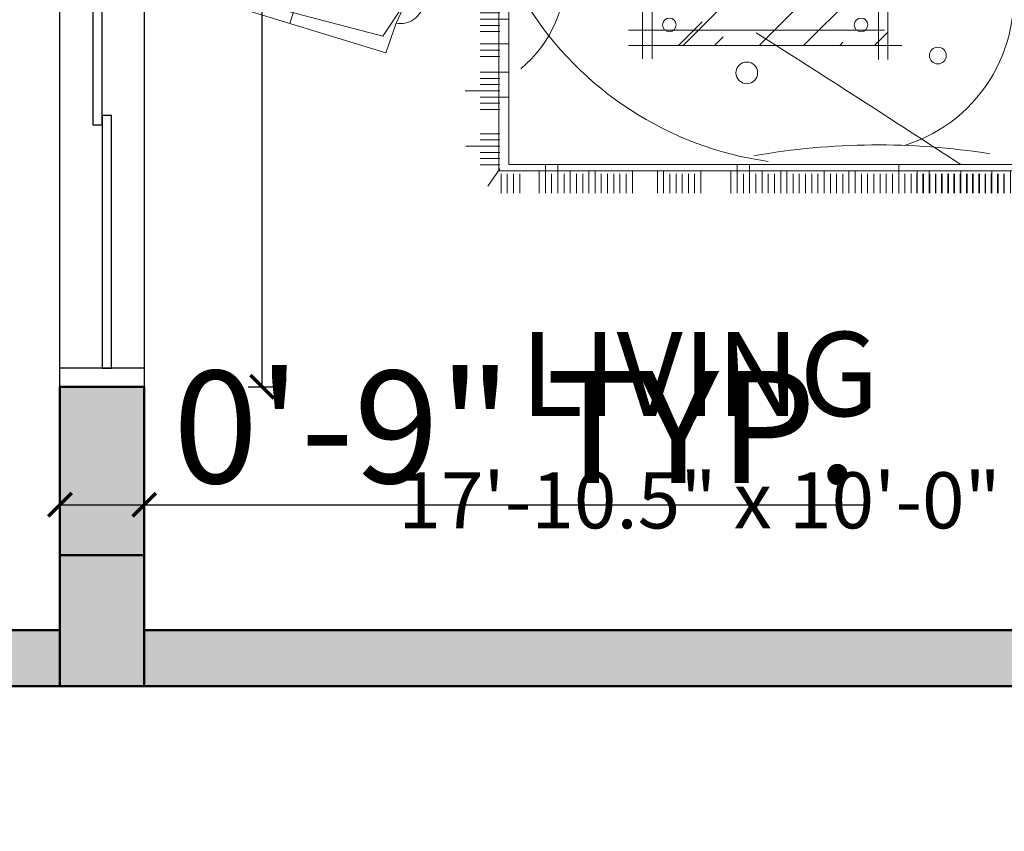
# Model space of a CAD drawing. Units: inches. Extents: x 375 to 1122, y 27 to 1069.
# Tile 4 of 155: x 494 to 599, y 313 to 400. Entities that reach past the tile are written whole.
import ezdxf

# ---------------------------------------------------------------- set-up
doc = ezdxf.new("R2010")
doc.units = ezdxf.units.IN
for name, color, linetype, lineweight in [('A-ANNO-DIMS', 2, 'Continuous', 18), ('A-AREA-IDEN', 7, 'Continuous', 18), ('A-COLS-PATT', 10, 'Continuous', 13), ('A-WALL-PATT', 252, 'Continuous', 13), ('Columns', 10, 'Continuous', 50), ('Doors', 150, 'Continuous', 25), ('Furniture', 30, 'Continuous', 18), ('Walls', 250, 'Continuous', 50)]:
    doc.layers.add(name, color=color, linetype=linetype, lineweight=lineweight)
doc.styles.get("Standard").update_dxf_attribs({"font": 'arial.ttf'})
doc.dimstyles.new('ISO-25', dxfattribs={"dimtxt": 12, "dimasz": 2.5, "dimexe": 1.5, "dimexo": 1.5, "dimtad": 1, "dimdec": 1, "dimlunit": 3, "dimtxsty": 'Standard', "dimblk": 'ARCHTICK', "dimcen": 2.5, "dimadec": 0, "dimazin": 0, "dimtfac": 1, "dimtdec": 1, "dimtmove": 0, "dimatfit": 3, "dimfxl": 1.5, "dimfxlon": 1, "dimarcsym": 0})

# ---------------------------------------------------------------- blocks, each defined once
blk = doc.blocks.new('A$C4DC51D13')
for p, q in [((3265.3, 2996.2), (1188.4, 2996.2)), ((1895.2, 2134), (1895.2, 2996.2)), ((2559.6, 2996.2), (2559.6, 2617.8)), ((1188.4, 2962.7), (1862.1, 2962.7)), ((1862.1, 2134), (1862.1, 2962.7)), ((1928.3, 2961.6), (2524.2, 2961.6)), ((1928.3, 2134), (1928.3, 2961.6)), ((2524.2, 2961.6), (2524.2, 2658.6)), ((2590.4, 2962.7), (2590.4, 2654.5)), ((3265.3, 2962.7), (2590.4, 2962.7)), ((277.4, 2939.6), (277.4, 2141.8)), ((943, 2103.5), (943, 2936.7)), ((1018.2, 2892.3), (232.2, 2892.3)), ((304, 2865.7), (304, 2253.3)), ((916.4, 2865.7), (304, 2865.7)), ((916.4, 2253.3), (916.4, 2865.7)), ((1290.4, 2664.8), (1028, 2870.9)), ((3163.3, 2664.8), (3425.7, 2870.9)), ((3778.5, 2897), (3631.2, 2747.3)), ((4008.9, 2375.5), (3778.5, 2897)), ((4156.2, 2525.2), (3778.5, 2897)), ((1022.9, 2163.8), (1022.9, 2830.3)), ((1056, 2830.3), (1081, 2194.8)), ((3397.7, 2830.3), (3364.5, 2194.8)), ((3430.8, 2163.8), (3430.8, 2830.3)), ((423.7, 2370.8), (776.6, 2723.7)), ((427.4, 2727.4), (772.8, 2367.1)), ((531.8, 2670.2), (531.8, 2717)), ((536, 2672.5), (536, 2718.7)), ((540.2, 2674.6), (540.2, 2720.2)), ((544.4, 2676.5), (544.4, 2721.6)), ((548.7, 2678.2), (548.7, 2722.9)), ((650.1, 2678.8), (650.1, 2723.3)), ((654.3, 2677.1), (654.3, 2722)), ((658.6, 2675.2), (658.6, 2720.7)), ((662.8, 2673.2), (662.8, 2719.2)), ((667, 2671), (667, 2717.6)), ((668.5, 2670.2), (668.5, 2717)), ((4008.9, 2375.5), (3631.2, 2747.3)), ((476.8, 2615), (476.8, 2682.5)), ((481, 2622.2), (481, 2686.2)), ((485.3, 2628.5), (485.3, 2689.7)), ((489.5, 2634.2), (489.5, 2693)), ((493.7, 2639.3), (493.7, 2696.1)), ((497.9, 2644), (497.9, 2699.1)), ((502.2, 2648.3), (502.2, 2701.8)), ((506.4, 2652.2), (506.4, 2704.4)), ((510.6, 2655.8), (510.6, 2706.9)), ((514.9, 2659.2), (514.9, 2709.2)), ((519.1, 2662.3), (519.1, 2711.3)), ((523.3, 2665.1), (523.3, 2713.4)), ((527.5, 2667.8), (527.5, 2715.2)), ((671.2, 2668.6), (671.2, 2715.9)), ((672.7, 2667.8), (672.7, 2715.2)), ((675.5, 2666.1), (675.5, 2714)), ((676.9, 2665.1), (676.9, 2713.4)), ((679.7, 2663.3), (679.7, 2712)), ((681.1, 2662.3), (681.1, 2711.3)), ((683.9, 2660.3), (683.9, 2709.9)), ((685.4, 2659.2), (685.4, 2709.2)), ((688.1, 2657), (688.1, 2707.7)), ((689.6, 2655.8), (689.6, 2706.9)), ((692.4, 2653.5), (692.4, 2705.3)), ((693.8, 2652.2), (693.8, 2704.4)), ((696.6, 2649.6), (696.6, 2702.7)), ((698, 2648.3), (698, 2701.8)), ((700.8, 2645.5), (700.8, 2700)), ((702.3, 2644), (702.3, 2699.1)), ((705, 2641), (705, 2697.2)), ((706.5, 2639.3), (706.5, 2696.1)), ((709.3, 2636), (709.3, 2694.1)), ((710.7, 2634.2), (710.7, 2693)), ((713.5, 2630.5), (713.5, 2690.9)), ((714.9, 2628.5), (714.9, 2689.7)), ((717.7, 2624.4), (717.7, 2687.4)), ((719.2, 2622.2), (719.2, 2686.2)), ((722, 2617.6), (722, 2683.8)), ((723.4, 2615), (723.4, 2682.5)), ((726.2, 2609.7), (726.2, 2679.9)), ((446.1, 2646.1), (500, 2646.1)), ((447.2, 2446.7), (447.2, 2647.8)), ((448.9, 2650.4), (504.4, 2650.4)), ((451.5, 2440.6), (451.5, 2654)), ((451.9, 2654.6), (509.2, 2654.6)), ((455.1, 2658.8), (514.4, 2658.8)), ((455.7, 2434.9), (455.7, 2659.6)), ((458.4, 2663.1), (520.2, 2663.1)), ((459.9, 2558.8), (459.9, 2664.9)), ((462, 2667.3), (526.7, 2667.3)), ((464.1, 2583.3), (464.1, 2669.7)), ((465.8, 2671.5), (534.1, 2671.5)), ((468.4, 2596.6), (468.4, 2674.3)), ((469.8, 2675.7), (542.8, 2675.7)), ((472.6, 2606.7), (472.6, 2678.5)), ((489.5, 2667.3), (489.5, 2633.5)), ((657.4, 2675.7), (730.4, 2675.7)), ((734.5, 2671.5), (666.1, 2671.5)), ((666.1, 2671.5), (734.5, 2671.5)), ((738.2, 2667.3), (673.5, 2667.3)), ((673.5, 2667.3), (738.2, 2667.3)), ((741.8, 2663.1), (680, 2663.1)), ((680, 2663.1), (741.8, 2663.1)), ((745.2, 2658.8), (685.8, 2658.8)), ((685.8, 2658.8), (745.2, 2658.8)), ((748.3, 2654.6), (691, 2654.6)), ((691, 2654.6), (748.3, 2654.6)), ((751.3, 2650.4), (695.8, 2650.4)), ((695.8, 2650.4), (751.3, 2650.4)), ((754.1, 2646.1), (700.2, 2646.1)), ((700.2, 2646.1), (754.1, 2646.1)), ((727.6, 2606.7), (727.6, 2678.5)), ((730.4, 2600.3), (730.4, 2675.7)), ((731.9, 2596.6), (731.9, 2674.3)), ((734.6, 2588.4), (734.6, 2671.3)), ((736.1, 2583.3), (736.1, 2669.7)), ((738.9, 2570.4), (738.9, 2666.6)), ((740.3, 2558.8), (740.3, 2664.9)), ((743.1, 2433.1), (743.1, 2661.5)), ((744.5, 2434.9), (744.5, 2659.6)), ((747.3, 2438.6), (747.3, 2656)), ((748.8, 2440.6), (748.8, 2654)), ((751.5, 2444.5), (751.5, 2650)), ((753, 2446.7), (753, 2647.8)), ((755.8, 2451.1), (755.8, 2643.5)), ((1283.3, 2574.2), (1290.4, 2664.8)), ((1290.4, 2664.8), (1894.7, 2664.8)), ((1895.2, 2663.7), (2557.3, 2663.7)), ((2603.6, 2664.8), (2559, 2664.8)), ((3163.3, 2664.8), (2764.7, 2664.8)), ((3170.4, 2574.2), (3163.3, 2664.8)), ((3631.7, 2676.6), (3938.2, 2375)), ((427.5, 2608.1), (473.3, 2608.1)), ((429.1, 2612.3), (475.4, 2612.3)), ((430.3, 2479), (430.3, 2615.5)), ((430.7, 2616.6), (477.7, 2616.6)), ((432.5, 2620.8), (480.2, 2620.8)), ((434.5, 2469.3), (434.5, 2625.2)), ((434.5, 2625), (482.9, 2625)), ((436.5, 2629.2), (485.8, 2629.2)), ((438.7, 2633.5), (488.9, 2633.5)), ((438.8, 2460.9), (438.8, 2633.6)), ((441, 2637.7), (492.3, 2637.7)), ((443, 2453.4), (443, 2641.1)), ((443.5, 2641.9), (496, 2641.9)), ((756.7, 2641.9), (704.2, 2641.9)), ((704.2, 2641.9), (756.7, 2641.9)), ((759.2, 2637.7), (707.9, 2637.7)), ((707.9, 2637.7), (759.2, 2637.7)), ((761.5, 2633.5), (711.3, 2633.5)), ((711.3, 2633.5), (761.5, 2633.5)), ((763.7, 2629.2), (714.4, 2629.2)), ((714.4, 2629.2), (763.7, 2629.2)), ((765.8, 2625), (717.3, 2625)), ((767.7, 2620.8), (720, 2620.8)), ((769.5, 2616.6), (722.5, 2616.6)), ((771.1, 2612.3), (724.8, 2612.3)), ((772.7, 2608.1), (726.9, 2608.1)), ((757.2, 2453.4), (757.2, 2641.1)), ((760, 2458.3), (760, 2636.3)), ((761.4, 2460.9), (761.4, 2633.6)), ((764.2, 2466.3), (764.2, 2628.2)), ((765.7, 2469.3), (765.7, 2625.2)), ((1798, 2530.2), (1812.1, 2637.9)), ((418.5, 2570.1), (461.3, 2570.1)), ((419.1, 2574.3), (462.1, 2574.3)), ((419.8, 2578.5), (462.9, 2578.5)), ((420.6, 2582.7), (464, 2582.7)), ((421.5, 2587), (465.2, 2587)), ((422.5, 2591.2), (466.5, 2591.2)), ((423.6, 2595.4), (467.9, 2595.4)), ((424.8, 2599.7), (469.6, 2599.7)), ((426.1, 2603.9), (471.3, 2603.9)), ((426.1, 2490.7), (426.1, 2603.9)), ((774.1, 2603.9), (728.9, 2603.9)), ((775.4, 2599.7), (730.7, 2599.7)), ((776.6, 2595.4), (732.3, 2595.4)), ((777.7, 2591.2), (733.7, 2591.2)), ((778.7, 2587), (735.1, 2587)), ((779.6, 2582.7), (736.2, 2582.7)), ((780.4, 2578.5), (737.3, 2578.5)), ((781.1, 2574.3), (738.2, 2574.3)), ((781.7, 2570.1), (738.9, 2570.1)), ((1895.5, 2582.2), (1932.3, 2494.6)), ((417.1, 2548.9), (459.4, 2548.9)), ((417.1, 2544.7), (459.5, 2544.7)), ((417.2, 2553.2), (459.6, 2553.2)), ((417.2, 2540.5), (459.6, 2540.5)), ((417.4, 2557.4), (459.8, 2557.4)), ((417.5, 2536.3), (459.9, 2536.3)), ((417.7, 2561.6), (460.2, 2561.6)), ((417.8, 2532), (460.3, 2532)), ((418.1, 2565.8), (460.7, 2565.8)), ((459.9, 2429.7), (459.9, 2535.7)), ((782.2, 2565.8), (739.6, 2565.8)), ((782.5, 2532), (740, 2532)), ((782.5, 2561.6), (740.1, 2561.6)), ((740.3, 2429.7), (740.3, 2535.7)), ((782.8, 2557.4), (740.4, 2557.4)), ((782.8, 2536.3), (740.4, 2536.3)), ((783, 2540.5), (740.6, 2540.5)), ((783, 2553.2), (740.7, 2553.2)), ((783.1, 2548.9), (740.8, 2548.9)), ((783.1, 2544.7), (740.8, 2544.7)), ((1022.9, 2554.4), (1249.6, 2554.4)), ((2559, 2535.8), (2557.3, 2535.8)), ((3430.8, 2554.4), (3204.1, 2554.4)), ((418.2, 2527.8), (460.8, 2527.8)), ((418.7, 2523.6), (461.4, 2523.6)), ((419.3, 2519.4), (462.2, 2519.4)), ((781, 2519.4), (738, 2519.4)), ((781.6, 2523.6), (738.8, 2523.6)), ((782.1, 2527.8), (739.4, 2527.8)), ((1200, 2520.5), (1251.9, 2440.8)), ((3253.7, 2520.5), (3201.8, 2440.8)), ((4008.9, 2375.5), (4156.2, 2525.2)), ((1243.2, 2146.7), (1272.2, 2431.8)), ((3210.5, 2146.7), (3181.5, 2431.8)), ((304, 2253.3), (916.4, 2253.3)), ((242.9, 2226.7), (1018.2, 2226.7)), ((1145.1, 2159.3), (1022.9, 2163.8)), ((1081, 2194.8), (1243.2, 2146.7)), ((1145.1, 2159.3), (1243.2, 2146.7)), ((2590.4, 2164.3), (2590.4, 2134)), ((3364.5, 2194.8), (3210.5, 2146.7)), ((3308.6, 2159.3), (3210.5, 2146.7)), ((3308.6, 2159.3), (3430.8, 2163.8)), ((498.8, 1837.1), (382.1, 2139.5)), ((1040.3, 1942.9), (421.2, 2132.6)), ((1244.8, 2113), (1243.2, 2146.7)), ((3208.9, 2113), (3210.5, 2146.7)), ((411.8, 2101.9), (992.6, 1890.2)), ((1839.5, 2113), (1244.8, 2113)), ((2308.5, 2111.9), (1950.4, 2111.9)), ((2614.2, 2113), (3208.9, 2113)), ((677.4, 2054.1), (612.9, 1843.6)), ((1839.5, 2079.9), (1244.8, 2079.9)), ((2322.1, 2078.8), (1950.4, 2078.8)), ((2614.2, 2079.9), (3208.9, 2079.9)), ((220.3, 2026), (19.3, 1370.1)), ((251.1, 2016.6), (37.1, 1314.7)), ((1009.7, 1828.1), (1040.3, 1942.9)), ((658.5, 1880), (717.8, 1809.1)), ((992.6, 1890.2), (993.4, 1733.4)), ((498.8, 1837.1), (341.4, 1323.6)), ((584.9, 1817.9), (498.8, 1837.1)), ((1009.7, 1828.1), (993.4, 1733.4)), ((1158.3, 1784.3), (1158.3, 1858.2)), ((1181.8, 1784.3), (1181.8, 1858.2)), ((1205.3, 1784.3), (1205.3, 1858.2)), ((1228.8, 1784.3), (1228.8, 1858.2)), ((1252.2, 1784.3), (1252.2, 1858.2)), ((1319.4, 1784.3), (1319.4, 1858.2)), ((1342.9, 1784.3), (1342.9, 1858.2)), ((1366.3, 1784.3), (1366.3, 1858.2)), ((1389.8, 1784.3), (1389.8, 1858.2)), ((1413.3, 1784.3), (1413.3, 1858.2)), ((1436.8, 1784.3), (1436.8, 1858.2)), ((1460.2, 1784.3), (1460.2, 1858.2)), ((1483.7, 1784.3), (1483.7, 1858.2)), ((1507.2, 1784.3), (1507.2, 1858.2)), ((1530.7, 1784.3), (1530.7, 1858.2)), ((1554.1, 1784.3), (1554.1, 1858.2)), ((1577.6, 1784.3), (1577.6, 1858.2)), ((1714.2, 1784.3), (1714.2, 1858.2)), ((1737.6, 1784.3), (1737.6, 1858.2)), ((1761.1, 1784.3), (1761.1, 1858.2)), ((1784.6, 1784.3), (1784.6, 1858.2)), ((1808.1, 1784.3), (1808.1, 1858.2)), ((1831.5, 1784.3), (1831.5, 1858.2)), ((1855, 1784.3), (1855, 1858.2)), ((1878.5, 1784.3), (1878.5, 1858.2)), ((1902, 1784.3), (1902, 1858.2)), ((2050.7, 1784.3), (2050.7, 1858.2)), ((2074.2, 1784.3), (2074.2, 1858.2)), ((2097.7, 1784.3), (2097.7, 1858.2)), ((2121.1, 1784.3), (2121.1, 1858.2)), ((2144.6, 1784.3), (2144.6, 1858.2)), ((2168.1, 1784.3), (2168.1, 1858.2)), ((2191.6, 1782.4), (2191.6, 1856.3)), ((2215, 1785.7), (2215, 1832.3)), ((2238.5, 1785.1), (2238.5, 1859)), ((2262, 1784.3), (2262, 1858.2)), ((2285.4, 1784.3), (2285.4, 1858.2)), ((2543.7, 1784.3), (2543.7, 1858.2)), ((2567.1, 1784.3), (2567.1, 1858.2)), ((2590.6, 1784.3), (2590.6, 1858.2)), ((2614.1, 1784.3), (2614.1, 1858.2)), ((2661, 1784.3), (2661, 1858.2)), ((2684.5, 1784.3), (2684.5, 1858.2)), ((2708, 1772.3), (2708, 1858.2)), ((2731.5, 1784.3), (2731.5, 1858.2)), ((2754.9, 1784.3), (2754.9, 1858.2)), ((2778.4, 1784.3), (2778.4, 1858.2)), ((2801.9, 1784.3), (2801.9, 1858.2)), ((2825.4, 1784.3), (2825.4, 1858.2)), ((2848.8, 1784.3), (2848.8, 1858.2)), ((2872.3, 1784.3), (2872.3, 1858.2)), ((2895.8, 1784.3), (2895.8, 1858.2)), ((2919.3, 1784.3), (2919.3, 1858.2)), ((2942.7, 1784.3), (2942.7, 1858.2)), ((2966.2, 1744.8), (2966.2, 1858.2)), ((2989.7, 1784.3), (2989.7, 1858.2)), ((3013.2, 1772.3), (3013.2, 1858.2)), ((3036.6, 1784.3), (3036.6, 1858.2)), ((3060.1, 1784.3), (3060.1, 1858.2)), ((3083.6, 1784.3), (3083.6, 1858.2)), ((993.4, 1733.4), (720.4, 1787.6)), ((1166.1, 1769.7), (1091.8, 1794.5)), ((1158.3, 1821.3), (1158.5, 487.7)), ((1162.1, 1754.9), (1088.2, 1754.9)), ((3248.4, 1772.3), (1158.5, 1772.3)), ((3248.4, 487.7), (3248.4, 1772.3)), ((3248.8, 1760.8), (3322.7, 1760.8)), ((1024.2, 1722.3), (842.3, 1125.2)), ((873.1, 1115.8), (1055, 1712.9)), ((1024.2, 1722.3), (993.4, 1733.4)), ((1162.1, 1741.1), (1088.2, 1741.1)), ((1162.1, 1717.6), (1088.2, 1717.6)), ((1196, 511), (1196, 1744.8)), ((1196, 1744.8), (3215.6, 1744.8)), ((3215.6, 511), (3215.6, 1744.8)), ((3248.8, 1737.3), (3322.7, 1737.3)), ((3248.8, 1713.8), (3322.7, 1713.8)), ((3600.6, 1621.7), (3605.1, 1743.8)), ((3605.1, 1743.8), (4271.6, 1743.8)), ((3995.7, 1743.8), (3995.7, 1517.1)), ((4106.1, 1476.4), (4312.2, 1738.8)), ((1162.1, 1708), (1088.2, 1708)), ((1162.1, 1684.5), (1088.2, 1684.5)), ((3248.8, 1690.4), (3322.7, 1690.4)), ((3636.1, 1685.8), (3588, 1523.6)), ((4271.6, 1710.7), (3636.1, 1685.8)), ((3248.8, 1666.9), (3322.7, 1666.9)), ((3248.8, 1643.4), (3322.7, 1643.4)), ((3248.8, 1619.9), (3322.7, 1619.9)), ((3600.6, 1621.7), (3588, 1523.6)), ((4404, 1578.3), (4404, 904.6)), ((4437.5, 165.9), (4437.5, 1578.3)), ((1701.7, 1530), (1701.7, 911.2)), ((1162.1, 1492.9), (1088.2, 1492.9)), ((2593.1, 907.9), (2593.1, 1490.3)), ((2629.1, 907.9), (2629.1, 1503.1)), ((3248.8, 1513.8), (3322.7, 1513.8)), ((3248.8, 1513.3), (3322.7, 1513.3)), ((3248.8, 1490.4), (3322.7, 1490.4)), ((3248.8, 1489.9), (3322.7, 1489.9)), ((3521.2, 1130.7), (3521.2, 1521.9)), ((3554.3, 1131.4), (3554.3, 1521.9)), ((3588, 1523.6), (3873.1, 1494.5)), ((1162.1, 1483.3), (1088.2, 1483.3)), ((1162.1, 1459.8), (1088.2, 1459.8)), ((1737.7, 1483.1), (1737.7, 911.2)), ((3248.8, 1466.9), (3322.7, 1466.9)), ((4015.5, 1483.4), (4106.1, 1476.4)), ((4106.1, 1476.4), (4106.1, 872.1)), ((1162.1, 1446), (1088.2, 1446)), ((2674.6, 1449.9), (1641, 1449.9)), ((1888.1, 1449.9), (1701.7, 1263.5)), ((1856.2, 1449.9), (1701.7, 1295.4)), ((1715.1, 1449.9), (1701.7, 1436.5)), ((2343.3, 1449.9), (1855.3, 961.9)), ((2629.1, 1449), (2142, 961.9)), ((2325.1, 1449.9), (2154.2, 1279.1)), ((2461.6, 1449.9), (2177, 1165.3)), ((3248.8, 1443.4), (3322.7, 1443.4)), ((3248.8, 1419.9), (3322.7, 1419.9)), ((1162.1, 1412.8), (1088.2, 1412.8)), ((1162.1, 1399), (1088.2, 1399)), ((2674.6, 1413.9), (1641, 1413.9)), ((3250, 1407.8), (3519, 1407.8)), ((6.3, 1324.2), (19.3, 1370.2)), ((479.3, 1327.3), (375.2, 1344.9)), ((1162.1, 1375.5), (1088.2, 1375.5)), ((1162.1, 1352.1), (1088.2, 1352.1)), ((1162.1, 1342.9), (1088.2, 1342.9)), ((1162.1, 1342.4), (1088.2, 1342.4)), ((3248.8, 1359), (3322.7, 1359)), ((342.8, 1324.6), (76.7, 1139.6)), ((843, 1127.6), (342.8, 1324.6)), ((1162.1, 1319.4), (1088.2, 1319.4)), ((1162.1, 1318.9), (1088.2, 1318.9)), ((3248.8, 990.8), (3248.4, 1328.4)), ((3248.8, 1312.1), (3322.7, 1312.1)), ((3250, 1317.8), (3519, 1317.8)), ((369.2, 1044.8), (442.9, 1285.2)), ((1162.1, 1296), (1088.2, 1296)), ((1162.1, 1295.5), (1088.2, 1295.5)), ((1196, 1272.5), (1088.2, 1272.5)), ((1162.1, 1272), (1088.2, 1272)), ((2629.1, 1280.5), (2310.5, 961.9)), ((3248.8, 1302.3), (3322.7, 1302.3)), ((1162.1, 1249), (1088.2, 1249)), ((1162.1, 1248.5), (1088.2, 1248.5)), ((3248.8, 1249), (3322.7, 1249)), ((3248.8, 1248.5), (3322.7, 1248.5)), ((3248.8, 1239.3), (3322.7, 1239.3)), ((3248.8, 1238.8), (3322.7, 1238.8)), ((1162.1, 1225.5), (1088.2, 1225.5)), ((1162.1, 1202.1), (1088.2, 1202.1)), ((3248.8, 1225.5), (3322.7, 1225.5)), ((3248.8, 1202.1), (3322.7, 1202.1)), ((122.4, 1154.1), (719.7, 996.3)), ((1196, 1178.6), (1088.2, 1178.6)), ((1162.1, 1155.1), (1088.2, 1155.1)), ((1728.6, 1158.4), (1701.7, 1131.5)), ((3248.8, 1178.6), (3322.7, 1178.6)), ((3248.8, 1155.1), (3322.7, 1155.1)), ((732, 933.5), (112.9, 1123.3)), ((719.7, 996.3), (810.6, 1133.2)), ((771, 1045.7), (810.6, 1133.2)), ((842.3, 1125.2), (810.6, 1133.2)), ((1162.1, 1131.6), (1088.2, 1131.6)), ((3248.8, 1131.6), (3322.7, 1131.6)), ((1162.1, 1108.2), (1088.2, 1108.2)), ((1162.1, 1084.7), (1088.2, 1084.7)), ((3248.8, 1108.2), (3322.7, 1108.2)), ((771, 1045.7), (732, 933.5)), ((1196, 1061.2), (1088.2, 1061.2)), ((1926.6, 1051.5), (1837.1, 961.9)), ((1162.1, 1037.7), (1088.2, 1037.7)), ((1162.1, 1014.3), (1088.2, 1014.3)), ((1648.3, 1019.6), (2616.7, 1019.6)), ((2629.1, 1012), (2579, 961.9)), ((3248.8, 1014.3), (3322.7, 1014.3)), ((2006.3, 994.6), (1973.6, 961.9)), ((2459.2, 974.1), (2447, 961.9)), ((3248.8, 990.8), (3322.7, 990.8)), ((1196, 967.3), (1088.2, 967.3)), ((1162.1, 943.8), (1088.2, 943.8)), ((1648.3, 961.9), (2681.9, 961.9)), ((3248.8, 967.3), (3322.7, 967.3)), ((3248.8, 943.8), (3322.7, 943.8)), ((1162.1, 920.4), (1088.2, 920.4)), ((3248.8, 920.4), (3322.7, 920.4)), ((4097.4, 904.6), (4404, 904.6)), ((1196, 860.5), (1088.2, 860.5)), ((4106.1, 871.5), (4437.5, 871.5)), ((1162.1, 837), (1088.2, 837)), ((4404, 840.7), (4110.5, 840.7)), ((4404, 165.9), (4404, 840.7)), ((1162.1, 790), (1031.8, 790)), ((1162.1, 813.5), (1088.2, 813.5)), ((3521.2, 816.9), (3521.2, 222.3)), ((3554.3, 816.9), (3554.3, 222.3)), ((1196, 766.6), (1088.2, 766.6)), ((1162.1, 743.1), (1088.2, 743.1)), ((1162.1, 719.6), (1088.2, 719.6)), ((4106.1, 267.8), (4106.1, 666.5)), ((1162.1, 627.8), (1088.2, 627.8)), ((1162.1, 604.4), (1088.2, 604.4)), ((3248.8, 627.8), (3322.7, 627.8)), ((3248.8, 604.4), (3322.7, 604.4)), ((1162.1, 580.9), (1034.2, 580.9)), ((3248.8, 580.9), (3322.7, 580.9)), ((1162.1, 557.4), (1088.2, 557.4)), ((1162.1, 533.9), (1088.2, 533.9)), ((3248.8, 557.4), (3322.7, 557.4)), ((3248.8, 533.9), (3322.7, 533.9)), ((1162.1, 510.5), (1088.2, 510.5)), ((1162, 495.1), (1116.6, 429)), ((1158.5, 487.7), (3248.4, 487.7)), ((3215.6, 511), (1196, 511)), ((1311.1, 487.7), (1311.1, 402.4)), ((1334.6, 511), (1334.6, 402.4)), ((1381.6, 511), (1381.6, 402.4)), ((1428.5, 487.7), (1428.5, 402.4)), ((1498.9, 487.7), (1498.9, 402.4)), ((1522.4, 487.7), (1522.4, 402.4)), ((1663.3, 487.7), (1663.3, 402.4)), ((1757.8, 487.7), (1757.8, 402.4)), ((1781.3, 487.7), (1781.3, 402.4)), ((1922.1, 487.7), (1922.1, 402.4)), ((2036, 487.7), (2036, 402.4)), ((2059.5, 511), (2059.5, 402.4)), ((2106.4, 511), (2106.4, 402.4)), ((2153.4, 487.7), (2153.4, 402.4)), ((2223.8, 487.7), (2223.8, 402.4)), ((2247.2, 487.7), (2247.2, 402.4)), ((2388.1, 487.7), (2388.1, 402.4)), ((2482, 487.7), (2482, 402.4)), ((2505.5, 487.7), (2505.5, 402.4)), ((2669.8, 511), (2669.8, 402.4)), ((2740.2, 487.7), (2740.2, 402.4)), ((2784.9, 487.7), (2784.9, 402.4)), ((2904.5, 487.7), (2904.5, 402.4)), ((3021.9, 487.7), (3021.9, 402.4)), ((3092.7, 484.5), (3092.7, 410.6)), ((3116.2, 484.5), (3116.2, 410.6)), ((3244.9, 495.1), (3290.3, 429)), ((3248.8, 510.5), (3322.7, 510.5)), ((1167.1, 476.3), (1167.1, 402.4)), ((1190.6, 476.3), (1190.6, 402.4)), ((1214, 476.3), (1214, 402.4)), ((1237.5, 476.3), (1237.5, 402.4)), ((1358.1, 476.3), (1358.1, 402.4)), ((1405, 476.3), (1405, 402.4)), ((1452, 476.3), (1452, 402.4)), ((1475.5, 476.3), (1475.5, 402.4)), ((1545.9, 476.3), (1545.9, 402.4)), ((1569.4, 476.3), (1569.4, 402.4)), ((1592.8, 476.3), (1592.8, 402.4)), ((1616.3, 476.3), (1616.3, 402.4)), ((1639.8, 476.3), (1639.8, 402.4)), ((1804.8, 476.3), (1804.8, 402.4)), ((1828.2, 476.3), (1828.2, 402.4)), ((1851.7, 476.3), (1851.7, 402.4)), ((1875.2, 476.3), (1875.2, 402.4)), ((1898.7, 476.3), (1898.7, 402.4)), ((2082.9, 476.3), (2082.9, 402.4)), ((2129.9, 476.3), (2129.9, 402.4)), ((2176.8, 476.3), (2176.8, 402.4)), ((2200.3, 476.3), (2200.3, 402.4)), ((2270.7, 476.3), (2270.7, 402.4)), ((2294.2, 476.3), (2294.2, 402.4)), ((2317.7, 476.3), (2317.7, 402.4)), ((2341.1, 476.3), (2341.1, 402.4)), ((2364.6, 476.3), (2364.6, 402.4)), ((2411.6, 476.3), (2411.6, 402.4)), ((2435, 476.3), (2435, 402.4)), ((2458.5, 476.3), (2458.5, 402.4)), ((2528.9, 476.3), (2528.9, 402.4)), ((2552.4, 476.3), (2552.4, 402.4)), ((2575.9, 476.3), (2575.9, 402.4)), ((2599.4, 476.3), (2599.4, 402.4)), ((2622.8, 476.3), (2622.8, 402.4)), ((2646.3, 476.3), (2646.3, 402.4)), ((2693.3, 476.3), (2693.3, 402.4)), ((2716.7, 476.3), (2716.7, 402.4)), ((2738, 476.3), (2738, 402.4)), ((2761.5, 476.3), (2761.5, 402.4)), ((2763.7, 476.3), (2763.7, 402.4)), ((2787.2, 476.3), (2787.2, 402.4)), ((2808.4, 476.3), (2808.4, 402.4)), ((2810.6, 476.3), (2810.6, 402.4)), ((2831.9, 476.3), (2831.9, 402.4)), ((2834.1, 476.3), (2834.1, 402.4)), ((2855.4, 476.3), (2855.4, 402.4)), ((2857.6, 476.3), (2857.6, 402.4)), ((2878.8, 476.3), (2878.8, 402.4)), ((2881.1, 476.3), (2881.1, 402.4)), ((2902.3, 476.3), (2902.3, 402.4)), ((2925.8, 476.3), (2925.8, 402.4)), ((2928, 476.3), (2928, 402.4)), ((2949.3, 476.3), (2949.3, 402.4)), ((2951.5, 476.3), (2951.5, 402.4)), ((2972.7, 476.3), (2972.7, 402.4)), ((2975, 476.3), (2975, 402.4)), ((2996.2, 476.3), (2996.2, 402.4)), ((2998.4, 476.3), (2998.4, 402.4)), ((3019.7, 476.3), (3019.7, 402.4)), ((3043.2, 476.3), (3043.2, 402.4)), ((3045.4, 476.3), (3045.4, 402.4)), ((3066.6, 476.3), (3066.6, 402.4)), ((3068.9, 476.3), (3068.9, 402.4)), ((3092.3, 476.3), (3092.3, 402.4)), ((3115.8, 476.3), (3115.8, 402.4)), ((3202.2, 476.3), (3202.2, 402.4)), ((3225.7, 476.3), (3225.7, 402.4)), ((3249.2, 476.3), (3249.2, 402.4)), ((4015.5, 260.8), (4106.1, 267.8)), ((4106.1, 267.8), (4312.2, 5.4)), ((3588, 220.6), (3873.1, 249.7)), ((3961.8, 177.4), (3882.1, 229.3)), ((3995.7, 0.4), (3995.7, 227)), ((3636.1, 66.6), (3588, 220.6)), ((3600.6, 122.5), (3605.1, 0.4)), ((4271.6, 33.5), (3636.1, 66.6)), ((3605.1, 0.4), (4271.6, 0.4))]:
    blk.add_line(p, q)
at = {"linetype": 'ByBlock'}
for points in [[(2342.9, 1843.9), (2352.5, 1810.4), (2340.1, 1777.7), (2351.8, 1757), (2412.3, 1818), (2433.1, 1866.4), (2453.1, 1889.5), (2436, 1914.7), (2407.6, 1926.2), (2433.7, 1959.9), (2473.1, 2048.3), (2530.6, 2101.1), (2625.9, 2180.3), (2669, 2174.2), (2748.1, 2315.4), (2745.8, 2342.6), (2801.2, 2404.9), (2823.9, 2479.6), (2818.4, 2529.9), (2775.1, 2571.7), (2782.4, 2583.3), (2765.2, 2658.8), (2714.5, 2706.9), (2634.6, 2708.6), (2571.9, 2652.6), (2548.8, 2649.4), (2474, 2672.1), (2312.9, 2542.1), (2312.9, 2341.6), (2333.9, 2336.4), (2302, 2223.9), (2313.6, 2216.6), (2297.4, 2095.7), (2309.3, 2034.9), (2320.2, 1952), (2319.3, 1929.9), (2280.8, 1863.6), (2257.7, 1842.4), (2239.2, 1825.7), (2220.1, 1798.2), (2221.6, 1713.1), (2254.3, 1700.7), (2275.9, 1729.8), (2288.6, 1768), (2313.7, 1797.6)], [(3285.2, 1088.3), (3251.7, 1078.6), (3219, 1091.1), (3198.3, 1079.4), (3259.3, 1018.8), (3307.7, 998), (3330.8, 978), (3356, 995.1), (3367.5, 1023.6), (3401.2, 997.5), (3489.6, 958), (3542.4, 900.5), (3621.6, 805.3), (3615.5, 762.2), (3756.7, 683), (3783.9, 685.3), (3846.2, 629.9), (3920.9, 607.2), (3971.2, 612.7), (4013, 656), (4024.6, 648.7), (4100.1, 665.9), (4148.2, 716.6), (4149.9, 796.5), (4093.9, 859.3), (4090.7, 882.4), (4113.4, 957.1), (3983.4, 1118.2), (3782.9, 1118.2), (3777.7, 1097.2), (3665.2, 1129.2), (3657.9, 1117.6), (3537, 1133.7), (3476.2, 1121.9), (3393.3, 1110.9), (3371.2, 1111.9), (3304.9, 1150.4), (3283.7, 1173.4), (3267, 1191.9), (3239.5, 1211), (3154.4, 1209.5), (3142, 1176.8), (3171.1, 1155.3), (3209.3, 1142.5), (3238.9, 1117.5)]]:
    blk.add_lwpolyline(points, close=True, dxfattribs=at)
for points in [[(2563.4, 2654.7), (2512.2, 2609.3), (2506.2, 2548.3), (2540.1, 2504.4), (2576.9, 2490.9), (2579.8, 2539.3), (2598.7, 2543.6), (2636.7, 2516.4), (2690.3, 2516.7), (2731.2, 2520.1), (2758.5, 2540.1), (2773, 2563.3)], [(2629.1, 2357.8), (2507, 2405.5), (2433.2, 2450.3), (2445.5, 2500.8), (2478.9, 2546.1), (2402.4, 2506.9), (2373.4, 2424.8), (2384.4, 2341.9), (2352.8, 2340.7)], [(2712.3, 2515.8), (2652.7, 2472.4), (2603.2, 2489), (2580, 2503.6)], [(2738, 2438.2), (2699.2, 2425.4), (2742.4, 2401.4), (2680.4, 2403.2), (2604.1, 2328.3), (2519.2, 2273.3), (2529.8, 2261.8), (2402.7, 2252.7), (2395.4, 2241.1), (2431.1, 2241.3), (2375.7, 2196.9), (2385.2, 2181.2), (2474.4, 2199.5), (2549.9, 2234.6), (2596.2, 2223.2), (2730.1, 2333.1)], [(2433.2, 2450.3), (2377.6, 2423.8)], [(2409.5, 2153), (2387.5, 2153.9), (2359, 2165.4), (2352.6, 2193.7), (2353.5, 2215.7), (2330.5, 2194.6), (2322.1, 2196.7), (2341.8, 2240.9), (2345.5, 2329.1)], [(2374.9, 2339.8), (2395.2, 2276.9)], [(2613.2, 2183.4), (2541.6, 2218.8)], [(2431.4, 2187.8), (2379.5, 2066.7), (2320.2, 1929.7)], [(2407.6, 1926.2), (2342.9, 1843.9)], [(2412.9, 1911.5), (2401.6, 1865.2), (2361.9, 1812.5)], [(2279.2, 1765.9), (2259.2, 1757.4), (2247.6, 1764.7), (2246.4, 1796.2), (2253.5, 1843.5)], [(3207.2, 1152), (3198.7, 1171.9), (3206, 1183.5), (3237.5, 1184.7), (3284.8, 1177.6)], [(3367.5, 1023.6), (3285.2, 1088.3)], [(3629.1, 999.7), (3508, 1051.6), (3371, 1110.9)], [(3594.3, 1021.6), (3595.2, 1043.7), (3606.7, 1072.1), (3635, 1078.6), (3657, 1077.6), (3635.9, 1100.6), (3638, 1109.1), (3682.2, 1089.3), (3770.4, 1085.6)], [(3352.8, 1018.2), (3306.5, 1029.5), (3253.8, 1069.2)], [(3879.5, 693.2), (3866.7, 732), (3842.7, 688.8), (3844.5, 750.8), (3769.6, 827.1), (3714.6, 911.9), (3703.1, 901.3), (3694, 1028.4), (3682.4, 1035.7), (3682.6, 1000), (3638.2, 1055.5), (3622.5, 1045.9), (3640.8, 956.7), (3675.9, 881.2), (3664.5, 834.9), (3774.4, 701)], [(3781.1, 1056.2), (3718.2, 1035.9)], [(3799.1, 802), (3846.8, 924.2), (3891.6, 998), (3942.1, 985.6), (3987.4, 952.2), (3948.2, 1028.7), (3866.1, 1057.7), (3783.2, 1046.8), (3782, 1078.3)], [(3891.6, 998), (3865.1, 1053.5)], [(4096, 867.7), (4050.6, 918.9), (3989.6, 924.9), (3945.7, 891.1), (3932.2, 854.2), (3980.6, 851.3), (3984.9, 832.4), (3957.7, 794.4), (3958, 740.9), (3961.4, 699.9), (3981.4, 672.7), (4004.6, 658.1)], [(3624.7, 817.9), (3660.1, 889.6)], [(3957.1, 718.8), (3913.7, 778.5), (3930.3, 827.9), (3944.9, 851.1)]]:
    blk.add_lwpolyline(points, dxfattribs=at)
for centre, radius in [((600.1, 2547.3), 183), ((600.1, 2547.3), 140.7), ((1803.2, 1372.6), 25.7), ((2527.6, 1372.6), 25.7), ((1803.2, 1039.3), 25.7), ((2527.6, 1039.3), 25.7), ((2817.9, 923.4), 31.7), ((2095.7, 858), 41)]:
    blk.add_circle(centre, radius)
for centre, radius, start, end in [((1188.4, 2830.3), 165.9, 90, 180), ((3265.3, 2830.3), 165.9, 0, 90), ((1188.4, 2830.3), 132.4, 90, 180), ((3265.3, 2830.3), 132.4, 0, 90), ((3666.8, 2712.2), 50, 135.4503, 225.4503), ((1626.8, 1949.8), 712.7, 74.928, 126.7929), ((1707.9, 1527), 1115.8, 84.6406, 117.0804), ((2192.2, 2032.6), 624.6, 69.4145, 118.3621), ((2633.9, 373.6), 2292.5, 91.8726, 91.9144), ((2832.8, 1963.1), 698.5, 52.9389, 95.0789), ((2210.2, 1780.8), 852.5, 76.866, 111.6839), ((2713.3, 1357.7), 1282.3, 65.0725, 87.2152), ((1459.9, 2882.7), 488.4, 244.7866, 313.8058), ((2216, 2892.1), 488.4, 234.4888, 282.1285), ((2993.8, 2882.7), 488.4, 248.2152, 295.2134), ((3973.2, 2410.6), 50, 225.4503, 315.4503), ((1234.5, 2169.3), 90, 186.4251, 276.5821), ((3219.2, 2169.3), 90, 263.4179, 353.5749), ((374.1, 1978.9), 160.8, 72.9571, 162.9571), ((1839.5, 2135.1), 22.1, 270, 0), ((1839.5, 2135.1), 55.2, 270, 0), ((1950.4, 2134), 55.2, 180, 270), ((1950.4, 2134), 22.1, 180, 270), ((2619.6, 2148.3), 68.5, 191.0595, 265.4426), ((2614.2, 2135.1), 22.1, 180, 270), ((374.1, 1978.9), 128.6, 72.9571, 162.9571), ((1584.7, 1047), 1245.7, 138.0296, 166.1636), ((1067.1, 1321), 692.3, 126.1642, 178.0291), ((974.8, 1747.9), 87.4, 336.375, 66.532), ((248.2, 1741.7), 474.4, 299.1514, 8.1705), ((4271.6, 1578.3), 165.9, 0, 90), ((4271.6, 1578.3), 132.4, 0, 90), ((944.2, 1233.8), 467.1, 309.4804, 56.621), ((3610.6, 1532.2), 90, 96.4251, 186.5821), ((3383, 1136.2), 721.4, 348.1046, 36.6442), ((2968.3, 1058.8), 1115.8, 356.7543, 27.0804), ((4324, 1306.8), 488.4, 154.7866, 202.7137), ((160.1, 1277), 160.8, 162.9571, 252.9571), ((160.1, 1277), 128.6, 162.9571, 252.9571), ((2517.5, 1143.6), 586.7, 287.3395, 13.1463), ((787.1, 1131.7), 87.4, 259.3822, 349.5393), ((2356.9, 1798.1), 1287.8, 212.1153, 261.9323), ((-29968.2, -49615.7), 59944, 56.743614, 57.623407), ((3404.4, 598.4), 698.5, 322.9389, 5.0789), ((2799, 717.9), 1282.3, 335.0725, 357.2152), ((4324, 437.4), 488.4, 158.2152, 205.2134), ((2591.9, -2109.1), 2694.5, 80.9842, 100.0261), ((3610.6, 212), 90, 173.4179, 263.5749), ((4271.6, 165.9), 132.4, 270, 0), ((4271.6, 165.9), 165.9, 270, 0)]:
    blk.add_arc(centre, radius, start, end)
blk = doc.blocks.new('BALCONY-SLIDER-3P-84IN')
for points in [[(0, 84), (9, 84), (9, 0), (0, 0)], [(2.5, 55), (3.5, 55), (3.5, 82), (2.5, 82)], [(3.5, 28), (4.5, 28), (4.5, 56.5), (3.5, 56.5)], [(4.5, 2), (5.5, 2), (5.5, 29), (4.5, 29)]]:
    blk.add_lwpolyline(points, close=True)
for points in [[(0, 82), (9, 82)], [(9, 2), (0, 2)]]:
    blk.add_lwpolyline(points)
blk = doc.blocks.new('COLUMN-14X9IN')
blk.add_lwpolyline([(0, 0), (14, 0), (14, 9), (0, 9)], close=True)
blk = doc.blocks.new('_ArchTick')
at = {"color": 0, "linetype": 'ByBlock', "const_width": 0.15}
blk.add_lwpolyline([(-0.5, -0.5), (0.5, 0.5)], dxfattribs=at)
blk = doc.blocks.new('*D71')
at = {"layer": 'A-ANNO-DIMS', "color": 0, "lineweight": -2, "transparency": 16777216}
for p, q in [((520.11, 444.53), (520.11, 661.17)), ((518.61, 444.53), (521.61, 444.53)), ((520.11, 360.53), (520.11, 444.53)), ((518.61, 360.53), (521.61, 360.53))]:
    blk.add_line(p, q, dxfattribs=at)
at = {"layer": 'Defpoints', "color": 0, "transparency": 16777216}
for p in [(507.51, 444.53), (520.11, 444.53), (507.51, 360.53)]:
    blk.add_point(p, dxfattribs=at)
at = {"layer": 'A-ANNO-DIMS', "color": 0, "lineweight": -2, "transparency": 16777216, "xscale": 2.5, "yscale": 2.5, "zscale": 2.5}
for p, rotation in [((520.11, 444.53), 90), ((520.11, 360.53), 270)]:
    blk.add_blockref('_ArchTick', p, dxfattribs=dict(at, rotation=rotation))
at = {"layer": 'A-ANNO-DIMS', "color": 0, "transparency": 16777216, "insert": (513.27, 554.1), "char_height": 12, "attachment_point": 5, "rotation": 90}
blk.add_mtext('3-PANEL SLIDER 7\'-0" TYP.', dxfattribs=at)
blk = doc.blocks.new('*D72')
at = {"layer": 'A-ANNO-DIMS', "color": 0, "lineweight": -2, "transparency": 16777216}
for p, q in [((498.51, 349.43), (498.51, 346.43)), ((507.51, 349.43), (507.51, 346.43)), ((498.51, 347.93), (507.51, 347.93)), ((507.51, 347.93), (584.4, 347.93))]:
    blk.add_line(p, q, dxfattribs=at)
at = {"layer": 'Defpoints', "color": 0, "transparency": 16777216}
for p in [(498.51, 360.53), (507.51, 360.53), (507.51, 347.93)]:
    blk.add_point(p, dxfattribs=at)
at = {"layer": 'A-ANNO-DIMS', "color": 0, "lineweight": -2, "transparency": 16777216, "xscale": 2.5, "yscale": 2.5, "zscale": 2.5, "rotation": 180}
blk.add_blockref('_ArchTick', (498.51, 347.93), dxfattribs=at)
at = {"layer": 'A-ANNO-DIMS', "color": 0, "lineweight": -2, "transparency": 16777216, "xscale": 2.5, "yscale": 2.5, "zscale": 2.5}
blk.add_blockref('_ArchTick', (507.51, 347.93), dxfattribs=at)
at = {"layer": 'A-ANNO-DIMS', "color": 0, "transparency": 16777216, "insert": (547.21, 354.68), "char_height": 12, "attachment_point": 5}
blk.add_mtext('0\'-9" TYP.', dxfattribs=at)
blk = doc.blocks.new('*D82')
at = {"layer": 'A-ANNO-DIMS', "color": 0, "lineweight": -2, "transparency": 16777216}
for p, q in [((401.51, 1009.53), (398.51, 1009.53)), ((400.01, 160.53), (400.01, 1009.53)), ((401.51, 160.53), (398.51, 160.53))]:
    blk.add_line(p, q, dxfattribs=at)
at = {"layer": 'Defpoints', "color": 0, "transparency": 16777216}
for p in [(400.01, 1009.53), (630.53, 1009.53), (630.53, 160.53)]:
    blk.add_point(p, dxfattribs=at)
at = {"layer": 'A-ANNO-DIMS', "color": 0, "lineweight": -2, "transparency": 16777216, "xscale": 2.5, "yscale": 2.5, "zscale": 2.5}
for p, rotation in [((400.01, 1009.53), 90), ((400.01, 160.53), 270)]:
    blk.add_blockref('_ArchTick', p, dxfattribs=dict(at, rotation=rotation))
at = {"layer": 'A-ANNO-DIMS', "color": 0, "transparency": 16777216, "insert": (393.26, 585.03), "char_height": 12, "attachment_point": 5, "rotation": 90}
blk.add_mtext('70\'-9"', dxfattribs=at)

msp = doc.modelspace()

# ---------------------------------------------------------------- hatches: boundary and pattern name
at = {"layer": 'A-COLS-PATT'}
h = msp.add_hatch(color=256, dxfattribs=at)
h.dxf.hatch_style = 1
h.paths.add_polyline_path([(512.51, 982.53), (498.51, 982.53), (498.51, 973.53), (512.51, 973.53)])
h.paths.add_polyline_path([(666.51, 982.53), (652.51, 982.53), (652.51, 973.53), (666.51, 973.53)])
h.paths.add_polyline_path([(802.01, 982.53), (788.01, 982.53), (788.01, 973.53), (802.01, 973.53)])
h.paths.add_polyline_path([(932.01, 982.53), (918.01, 982.53), (918.01, 973.53), (932.01, 973.53)])
h.paths.add_polyline_path([(507.51, 841.53), (498.51, 841.53), (498.51, 827.53), (507.51, 827.53)])
h.paths.add_polyline_path([(666.51, 844.53), (652.51, 844.53), (652.51, 835.53), (666.51, 835.53)])
h.paths.add_polyline_path([(802.01, 814.53), (788.01, 814.53), (788.01, 805.53), (802.01, 805.53)])
h.paths.add_polyline_path([(932.01, 814.53), (918.01, 814.53), (918.01, 805.53), (932.01, 805.53)])
h.paths.add_polyline_path([(507.51, 719.53), (498.51, 719.53), (498.51, 705.53), (507.51, 705.53)])
h.paths.add_polyline_path([(731.01, 676.53), (722.01, 676.53), (722.01, 662.53), (731.01, 662.53)])
h.paths.add_polyline_path([(802.01, 676.53), (788.01, 676.53), (788.01, 667.53), (802.01, 667.53)])
h.paths.add_polyline_path([(932.01, 676.53), (918.01, 676.53), (918.01, 667.53), (932.01, 667.53)])
h.paths.add_polyline_path([(932.01, 583.53), (918.01, 583.53), (918.01, 574.53), (932.01, 574.53)])
h.paths.add_polyline_path([(868.01, 583.53), (854.01, 583.53), (854.01, 574.53), (868.01, 574.53)])
h.paths.add_polyline_path([(868.01, 502.53), (854.01, 502.53), (854.01, 493.53), (868.01, 493.53)])
h.paths.add_polyline_path([(932.01, 502.53), (918.01, 502.53), (918.01, 493.53), (932.01, 493.53)])
h.paths.add_polyline_path([(672.51, 592.03), (663.51, 592.03), (663.51, 578.03), (672.51, 578.03)])
h.paths.add_polyline_path([(512.51, 589.53), (498.51, 589.53), (498.51, 580.53), (512.51, 580.53)])
h.paths.add_polyline_path([(507.51, 464.53), (498.51, 464.53), (498.51, 450.53), (507.51, 450.53)])
h.paths.add_polyline_path([(731.01, 507.53), (722.01, 507.53), (722.01, 493.53), (731.01, 493.53)])
h.paths.add_polyline_path([(802.01, 502.53), (788.01, 502.53), (788.01, 493.53), (802.01, 493.53)])
h.paths.add_polyline_path([(507.51, 342.53), (498.51, 342.53), (498.51, 328.53), (507.51, 328.53)])
h.paths.add_polyline_path([(512.51, 196.53), (498.51, 196.53), (498.51, 187.53), (512.51, 187.53)])
h.paths.add_polyline_path([(666.51, 334.53), (652.51, 334.53), (652.51, 325.53), (666.51, 325.53)])
h.paths.add_polyline_path([(666.51, 196.53), (652.51, 196.53), (652.51, 187.53), (666.51, 187.53)])
h.paths.add_polyline_path([(805.01, 196.53), (791.01, 196.53), (791.01, 187.53), (805.01, 187.53)])
h.paths.add_polyline_path([(932.01, 196.53), (918.01, 196.53), (918.01, 187.53), (932.01, 187.53)])
h.paths.add_polyline_path([(932.01, 334.53), (918.01, 334.53), (918.01, 325.53), (932.01, 325.53)])
h.paths.add_polyline_path([(805.01, 334.53), (791.01, 334.53), (791.01, 325.53), (805.01, 325.53)])
at = {"layer": 'A-WALL-PATT'}
h = msp.add_hatch(color=256, dxfattribs=at)
h.dxf.hatch_style = 1
h.paths.add_polyline_path([(962.01, 388.53), (989.01, 388.53), (989.01, 394.53), (962.01, 394.53), (932.01, 394.53), (932.01, 397.53), (923.01, 397.53), (923.01, 394.53), (842.01, 394.53), (842.01, 334.53), (839.51, 334.53), (839.51, 328.53), (854.01, 328.53), (854.01, 334.53), (848.01, 334.53), (848.01, 388.53), (953.01, 388.53), (953.01, 356.08), (962.01, 356.08), (962.01, 358.55), (989.01, 358.55), (989.01, 364.55), (962.01, 364.55)])
h.paths.add_polyline_path([(989.01, 502.53), (932.01, 502.53), (932.01, 583.53), (932.01, 593.53), (923.01, 593.53), (923.01, 583.53), (854.01, 583.53), (854.01, 556.53), (863.01, 556.53), (863.01, 574.53), (923.01, 574.53), (923.01, 502.53), (863.01, 502.53), (863.01, 520.53), (854.01, 520.53), (854.01, 502.53), (773.01, 502.53), (773.01, 493.53), (788.01, 493.53), (788.01, 402.03), (722.01, 402.03), (722.01, 373.53), (728.01, 373.53), (728.01, 396.03), (788.01, 396.03), (788.01, 373.53), (794.01, 373.53), (794.01, 430.53), (814.01, 430.53), (814.01, 436.53), (794.01, 436.53), (794.01, 493.53), (923.01, 493.53), (923.01, 487.53), (932.01, 487.53), (932.01, 493.53), (983.01, 493.53), (983.01, 473.53), (989.01, 473.53)])
h.paths.add_polyline_path([(797.01, 325.53), (805.01, 325.53), (805.01, 328.53), (807.51, 328.53), (807.51, 334.53), (791.01, 334.53), (791.01, 226.53), (770.76, 226.53), (770.76, 217.53), (791.01, 217.53), (791.01, 187.53), (855.01, 187.53), (855.01, 196.53), (797.01, 196.53)])
h.paths.add_polyline_path([(989.01, 238.53), (962.01, 238.53), (962.01, 256.42), (953.01, 256.42), (953.01, 229.53), (980.01, 229.53), (980.01, 196.53), (915.01, 196.53), (915.01, 187.53), (989.01, 187.53)])
h.paths.add_polyline_path([(962.01, 334.53), (884.01, 334.53), (884.01, 328.53), (918.01, 328.53), (918.01, 325.53), (932.01, 325.53), (932.01, 328.53), (953.01, 328.53), (953.01, 304.42), (962.01, 304.42)])
h.paths.add_polyline_path([(606.51, 283.53), (609.51, 283.53), (609.51, 289.53), (600.51, 289.53), (600.51, 196.53), (578.51, 196.53), (578.51, 187.53), (606.51, 187.53), (606.51, 196.53)])
h.paths.add_polyline_path([(666.51, 292.53), (660.51, 292.53), (660.51, 289.53), (633.51, 289.53), (633.51, 283.53), (660.51, 283.53), (660.51, 196.53), (628.01, 196.53), (628.01, 187.53), (630.53, 187.53), (630.53, 160.53), (636.53, 160.53), (636.53, 187.53), (660.51, 187.53), (660.51, 160.53), (666.51, 160.53), (666.51, 217.53), (686.76, 217.53), (686.76, 226.53), (666.51, 226.53)])
h.paths.add_polyline_path([(480.51, 256.42), (471.51, 256.42), (471.51, 238.53), (444.51, 238.53), (444.51, 187.53), (518.51, 187.53), (518.51, 196.53), (453.51, 196.53), (453.51, 229.53), (480.51, 229.53)])
h.paths.add_polyline_path([(480.51, 328.53), (652.51, 328.53), (652.51, 325.53), (660.51, 325.53), (660.51, 322.53), (666.51, 322.53), (666.51, 334.53), (507.51, 334.53), (507.51, 360.53), (498.51, 360.53), (498.51, 334.53), (471.51, 334.53), (471.51, 304.42), (480.51, 304.42)])
h.paths.add_polyline_path([(507.51, 484.53), (498.51, 484.53), (498.51, 444.53), (507.51, 444.53), (507.51, 454.53), (621.51, 454.53), (621.51, 460.53), (507.51, 460.53)])
h.paths.add_polyline_path([(672.51, 604.53), (683.26, 604.53), (683.26, 613.53), (669.51, 613.53), (669.51, 649.53), (663.51, 649.53), (663.51, 589.53), (507.51, 589.53), (507.51, 613.53), (498.51, 613.53), (498.51, 556.53), (507.51, 556.53), (507.51, 580.53), (663.51, 580.53), (663.51, 520.53), (669.51, 520.53), (669.51, 556.53), (683.26, 556.53), (683.26, 565.53), (672.51, 565.53)])
h.paths.add_polyline_path([(731.01, 667.53), (734.01, 667.53), (734.01, 676.53), (728.01, 676.53), (728.01, 715.53), (657.51, 715.53), (657.51, 709.53), (663.51, 709.53), (663.51, 673.53), (669.51, 673.53), (669.51, 709.53), (722.01, 709.53), (722.01, 613.53), (704.76, 613.53), (704.76, 604.53), (722.01, 604.53), (722.01, 565.53), (704.76, 565.53), (704.76, 556.53), (722.01, 556.53), (722.01, 502.53), (722.01, 460.53), (669.51, 460.53), (669.51, 496.53), (663.51, 496.53), (663.51, 460.53), (657.51, 460.53), (657.51, 454.53), (728.01, 454.53), (728.01, 493.53), (734.01, 493.53), (734.01, 502.53), (731.01, 502.53)])
h.paths.add_polyline_path([(986.01, 718.53), (959.01, 718.53), (959.01, 727.53), (950.01, 727.53), (950.01, 709.53), (977.01, 709.53), (977.01, 676.53), (794.01, 676.53), (794.01, 805.53), (802.01, 805.53), (802.01, 808.53), (804.51, 808.53), (804.51, 814.53), (788.01, 814.53), (788.01, 774.03), (728.01, 774.03), (728.01, 796.53), (722.01, 796.53), (722.01, 768.03), (788.01, 768.03), (788.01, 676.53), (773.01, 676.53), (773.01, 667.53), (923.01, 667.53), (923.01, 657.53), (932.01, 657.53), (932.01, 667.53), (986.01, 667.53)])
h.paths.add_polyline_path([(621.51, 715.53), (507.51, 715.53), (507.51, 733.53), (498.51, 733.53), (498.51, 715.53), (498.51, 685.53), (507.51, 685.53), (507.51, 709.53), (621.51, 709.53)])
h.paths.add_polyline_path([(666.51, 847.03), (660.51, 847.03), (660.51, 844.53), (652.51, 844.53), (652.51, 841.53), (480.51, 841.53), (480.51, 859.53), (471.51, 859.53), (471.51, 835.53), (498.51, 835.53), (498.51, 817.53), (507.51, 817.53), (507.51, 835.53), (666.51, 835.53)])
h.paths.add_polyline_path([(480.51, 940.53), (453.51, 940.53), (453.51, 973.53), (518.51, 973.53), (518.51, 982.53), (444.51, 982.53), (444.51, 931.53), (471.51, 931.53), (471.51, 907.53), (480.51, 907.53)])
h.paths.add_polyline_path([(606.51, 982.53), (578.51, 982.53), (578.51, 973.53), (600.51, 973.53), (600.51, 880.53), (609.51, 880.53), (609.51, 886.53), (606.51, 886.53)])
h.paths.add_polyline_path([(666.51, 943.53), (686.76, 943.53), (686.76, 952.53), (666.51, 952.53), (666.51, 1009.53), (660.51, 1009.53), (660.51, 982.53), (636.53, 982.53), (636.53, 1009.53), (630.53, 1009.53), (630.53, 982.53), (628.01, 982.53), (628.01, 973.53), (660.51, 973.53), (660.51, 886.53), (633.51, 886.53), (633.51, 880.53), (660.51, 880.53), (660.51, 877.03), (666.51, 877.03)])
h.paths.add_polyline_path([(986.01, 874.53), (932.01, 874.53), (932.01, 877.53), (923.01, 877.53), (923.01, 874.53), (788.01, 874.53), (788.01, 868.53), (788.01, 844.53), (794.01, 844.53), (794.01, 868.53), (839.01, 868.53), (839.01, 814.53), (836.51, 814.53), (836.51, 808.53), (851.01, 808.53), (851.01, 814.53), (845.01, 814.53), (845.01, 868.53), (986.01, 868.53)])
h.paths.add_polyline_path([(959.01, 838.55), (986.01, 838.55), (986.01, 844.55), (959.01, 844.55), (959.01, 847.03), (950.01, 847.03), (950.01, 814.53), (881.01, 814.53), (881.01, 808.53), (918.01, 808.53), (918.01, 805.53), (932.01, 805.53), (932.01, 808.53), (950.01, 808.53), (950.01, 793.53), (959.01, 793.53)])
h.paths.add_polyline_path([(986.01, 982.53), (899.01, 982.53), (899.01, 973.53), (923.01, 973.53), (923.01, 967.53), (932.01, 967.53), (932.01, 973.53), (980.01, 973.53), (980.01, 953.53), (986.01, 953.53)])
h.paths.add_polyline_path([(851.01, 982.53), (788.01, 982.53), (788.01, 952.53), (770.76, 952.53), (770.76, 943.53), (788.01, 943.53), (788.01, 910.53), (814.01, 910.53), (814.01, 916.53), (794.01, 916.53), (794.01, 973.53), (851.01, 973.53)])

# ---------------------------------------------------------------- linework, layer by layer
at = {"layer": 'Walls'}
for p, q in [((498.51, 334.53), (498.51, 360.53)), ((507.51, 360.53), (498.51, 360.53)), ((507.51, 334.53), (507.51, 360.53)), ((471.51, 334.53), (498.51, 334.53)), ((507.51, 334.53), (666.51, 334.53)), ((480.51, 328.53), (652.51, 328.53))]:
    msp.add_line(p, q, dxfattribs=at)

# ---------------------------------------------------------------- block references
at = {"layer": 'Columns', "rotation": 270}
msp.add_blockref('COLUMN-14X9IN', (498.51, 342.53), dxfattribs=at)
at = {"layer": 'Doors'}
msp.add_blockref('BALCONY-SLIDER-3P-84IN', (498.51, 360.53), dxfattribs=at)
at = {"layer": 'Furniture', "xscale": 0.0282665567793757, "yscale": 0.0282665567793757, "zscale": 0.0282665567793757}
msp.add_blockref('A$C4DC51D13', (512.64, 369.84), dxfattribs=at)

# ---------------------------------------------------------------- texts
at = {"layer": 'A-AREA-IDEN', "insert": (533.78, 366.4), "char_height": 12, "attachment_point": 1}
msp.add_mtext_dynamic_manual_height_columns('\\pxqc;{\\fArial|b1|i0|c0|p34;\\H0.75x;LIVING\\H1.33333x;\\P\\fArial|b0|i0|c0|p34;\\H0.5x;17\'-10.5" x 10\'-0"}', width=66.1169, gutter_width=12.5, heights=[0], dxfattribs=at)

# ---------------------------------------------------------------- dimensions: what is measured, and where the dimension line sits
at = {"layer": 'A-ANNO-DIMS'}
dim = msp.add_linear_dim(base=(400.01, 1009.53), p1=(630.53, 160.53), p2=(630.53, 1009.53), angle=90, dimstyle='ISO-25', override={"dimdec": 1, "dimlfac": 1, "dimrnd": 0, "dimzin": 1, "dimdsep": 46, "dimlunit": 4, "dimfrac": 2}, dxfattribs=at)
dim.commit()
dim.dimension.update_dxf_attribs({"geometry": '*D82', "text_midpoint": (393.26, 585.03)})
dim = msp.add_linear_dim(base=(520.11, 444.53), p1=(507.51, 360.53), p2=(507.51, 444.53), angle=90, text='3-PANEL SLIDER <> TYP.', dimstyle='ISO-25', override={"dimdec": 1, "dimlfac": 1, "dimrnd": 0, "dimzin": 1, "dimdsep": 46, "dimlunit": 4, "dimfrac": 2}, dxfattribs=at)
dim.commit()
dim.dimension.update_dxf_attribs({"geometry": '*D71', "text_midpoint": (513.27, 554.1)})
dim = msp.add_linear_dim(base=(507.51, 347.93), p1=(498.51, 360.53), p2=(507.51, 360.53), text='<> TYP.', dimstyle='ISO-25', override={"dimdec": 1, "dimlfac": 1, "dimrnd": 0, "dimzin": 1, "dimdsep": 46, "dimlunit": 4, "dimfrac": 2}, dxfattribs=at)
dim.commit()
dim.dimension.update_dxf_attribs({"geometry": '*D72', "text_midpoint": (547.21, 354.68)})

doc.saveas('drawing.dxf')
